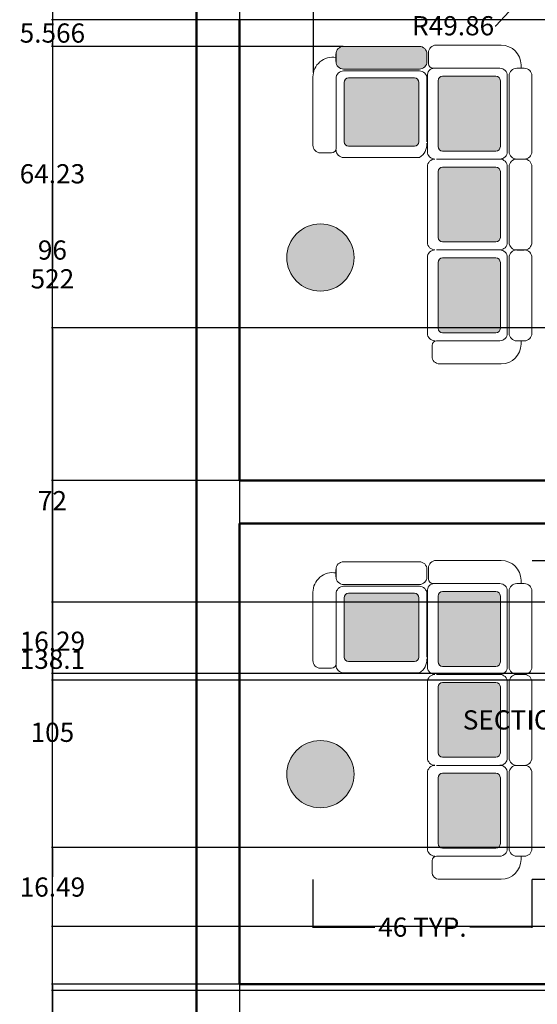
# Model space of a CAD drawing. Units: inches. Extents: x 1454 to 2136, y 626 to 1213.
# Tile 2 of 23: x 1456 to 1564, y 768 to 973. Entities that reach past the tile are written whole.
import ezdxf

# ---------------------------------------------------------------- set-up
doc = ezdxf.new("R2010")
doc.units = ezdxf.units.IN
doc.header["$MEASUREMENT"] = 0
for name, color, linetype, lineweight in [('A-ANNO-DIMS', 2, 'Continuous', 18), ('A-FURN', 9, 'Continuous', 18), ('A-FURN-PATT', 252, 'Continuous', 13), ('A-WALL', 7, 'Continuous', 50), ('sofa', 4, 'Continuous', 18)]:
    doc.layers.add(name, color=color, linetype=linetype, lineweight=lineweight)
doc.styles.get("Standard").update_dxf_attribs({"font": 'arial.ttf'})
doc.dimstyles.get("Standard").update_dxf_attribs({"dimtxt": 4, "dimasz": 0.18, "dimexe": 0.18, "dimexo": 0.0625, "dimgap": 0.09, "dimtad": 0, "dimtih": 1, "dimtoh": 1, "dimdec": 0, "dimrnd": 6, "dimzin": 0, "dimdsep": 46, "dimlunit": 3, "dimtxsty": 'Standard', "dimcen": 0.09, "dimadec": 0, "dimazin": 0, "dimtfac": 1, "dimtdec": 0, "dimtofl": 0, "dimtmove": 0, "dimatfit": 3, "dimfxl": 1, "dimtolj": 1, "dimtzin": 0, "dimarcsym": 0})

# ---------------------------------------------------------------- blocks, each defined once
blk = doc.blocks.new('A$C611E44E9')
for p, q in [((0.6611, 1.4447), (0.2101, 1.4447)), ((0.7111, 1.3223), (0.7111, 1.3947)), ((0.0084, 1.2424), (0.0084, 0.7424)), ((0.1084, 1.2927), (0.0584, 1.2927)), ((0.0584, 1.2924), (0.1084, 1.2924)), ((0.1584, 1.2424), (0.1584, 0.7424)), ((0.1705, 1.2422), (0.1705, 0.7424)), ((0.6811, 1.2924), (0.2205, 1.2924)), ((0.6811, 1.2924), (0.2205, 1.2924)), ((0.6811, 1.2922), (0.2205, 1.2922)), ((0.2465, 1.2392), (0.6374, 1.2392)), ((0.7418, 0.7424), (0.7418, 1.2422)), ((0.2165, 0.7749), (0.2165, 1.2092)), ((0.6674, 1.2092), (0.6674, 0.7749)), ((0.6374, 0.7449), (0.2465, 0.7449)), ((0.1224, 0.6827), (0.05, 0.6827)), ((0.1084, 0.6927), (0.0584, 0.6927)), ((0.0584, 0.6924), (0.1084, 0.6924)), ((0.1524, 0.6527), (0.1524, 0.2121)), ((0.2024, 0.6896), (0.7021, 0.6896)), ((0.6373, 0.6924), (0.2205, 0.6924)), ((0.6373, 0.6924), (0.2205, 0.6924)), ((0.8021, 0.6896), (1.3018, 0.6896)), ((1.4021, 0.6896), (1.9018, 0.6896)), ((1.982, 0.6589), (2.0543, 0.6589)), ((0, 0.6327), (0, 0.2017)), ((0.2048, 0.5892), (0.2048, 0.2381)), ((0.6691, 0.6192), (0.2348, 0.6192)), ((0.6991, 0.2381), (0.6991, 0.5892)), ((0.7521, 0.6289), (0.7521, 0.2121)), ((0.7521, 0.6289), (0.7521, 0.2121)), ((0.8045, 0.5892), (0.8045, 0.2381)), ((1.2688, 0.6192), (0.8345, 0.6192)), ((1.2988, 0.2381), (1.2988, 0.5892)), ((1.3521, 0.6289), (1.3521, 0.2121)), ((1.3521, 0.6289), (1.3521, 0.2121)), ((1.4045, 0.5892), (1.4045, 0.2381)), ((1.8688, 0.6192), (1.4345, 0.6192)), ((1.8988, 0.2381), (1.8988, 0.5892)), ((1.9518, 0.6289), (1.9518, 0.2121)), ((1.952, 0.6289), (1.952, 0.2121)), ((2.1043, 0.6089), (2.1043, 0.2017)), ((0.2348, 0.2081), (0.6691, 0.2081)), ((0.8345, 0.2081), (1.2688, 0.2081)), ((1.4345, 0.2081), (1.8688, 0.2081)), ((0.7021, 0.1621), (0.2024, 0.1621)), ((0.7024, 0.15), (0.2024, 0.15)), ((1.3018, 0.1621), (0.8021, 0.1621)), ((1.3021, 0.15), (0.8021, 0.15)), ((1.9018, 0.1621), (1.4021, 0.1621)), ((1.9021, 0.15), (1.4021, 0.15)), ((0.13, 0.0717), (0.15, 0.0717)), ((0.1524, 0.05), (0.1524, 0.1)), ((0.7521, 0.05), (0.7521, 0.1)), ((0.7524, 0.1), (0.7524, 0.05)), ((1.3521, 0.05), (1.3521, 0.1)), ((1.3524, 0.1), (1.3524, 0.05)), ((1.952, 0.05), (1.952, 0.1)), ((1.9521, 0.1), (1.9521, 0.05)), ((1.9743, 0.0717), (1.9543, 0.0717)), ((0.7024, 0), (0.2024, 0)), ((1.3021, 0), (0.8021, 0)), ((1.9021, 0), (1.4021, 0))]:
    blk.add_line(p, q)
for centre, radius, start, end in [((0.2101, 1.3147), 0.13, 90, 189.86144), ((0.6611, 1.3947), 0.05, 0, 90), ((0.6811, 1.3223), 0.03, 270, 0), ((0.0584, 1.2424), 0.05, 90, 180), ((0.1084, 1.2424), 0.05, 0, 90), ((0.2205, 1.2422), 0.05, 90, 180), ((0.2465, 1.2092), 0.03, 90, 180), ((0.6374, 1.2092), 0.03, 0, 90), ((0.6918, 1.2422), 0.05, 0, 90), ((0.0584, 0.7424), 0.05, 180, 270), ((0.1084, 0.7424), 0.05, 270, 0), ((0.2205, 0.7424), 0.05, 180, 270), ((0.2465, 0.7749), 0.03, 180, 270), ((0.6374, 0.7749), 0.03, 270, 0), ((0.653, 0.796), 0.1037, 267.24891, 328.87945), ((0.05, 0.6327), 0.05, 90, 180), ((0.1224, 0.6527), 0.03, 0, 90), ((0.1981, 0.6441), 0.0458, 84.66489, 178.99029), ((0.7021, 0.6396), 0.05, 0, 90), ((0.8021, 0.6396), 0.05, 90, 180), ((1.3018, 0.6396), 0.05, 0, 90), ((1.4021, 0.6396), 0.05, 90, 180), ((1.9018, 0.6396), 0.05, 0, 90), ((1.982, 0.6289), 0.03, 90, 180), ((2.0543, 0.6089), 0.05, 0, 90), ((0.2348, 0.5892), 0.03, 90, 180), ((0.6691, 0.5892), 0.03, 0, 90), ((0.8345, 0.5892), 0.03, 90, 180), ((1.2688, 0.5892), 0.03, 0, 90), ((1.4345, 0.5892), 0.03, 90, 180), ((1.8688, 0.5892), 0.03, 0, 90), ((0.13, 0.2017), 0.13, 180, 270), ((0.2024, 0.2121), 0.05, 180, 270), ((0.2348, 0.2381), 0.03, 180, 270), ((0.6691, 0.2381), 0.03, 270, 0), ((0.7021, 0.2121), 0.05, 270, 0), ((0.8021, 0.2121), 0.05, 180, 270), ((0.8345, 0.2381), 0.03, 180, 270), ((1.2688, 0.2381), 0.03, 270, 0), ((1.3018, 0.2121), 0.05, 270, 0), ((1.4021, 0.2121), 0.05, 180, 270), ((1.4345, 0.2381), 0.03, 180, 270), ((1.8688, 0.2381), 0.03, 270, 0), ((1.9018, 0.2121), 0.05, 270, 0), ((1.9743, 0.2017), 0.13, 270, 0), ((0.2024, 0.1), 0.05, 90, 180), ((0.7024, 0.1), 0.05, 0, 90), ((0.8021, 0.1), 0.05, 90, 180), ((1.3021, 0.1), 0.05, 0, 90), ((1.4021, 0.1), 0.05, 90, 180), ((1.9021, 0.1), 0.05, 0, 90), ((0.2024, 0.05), 0.05, 180, 270), ((0.7024, 0.05), 0.05, 270, 0), ((0.8021, 0.05), 0.05, 180, 270), ((1.3021, 0.05), 0.05, 270, 0), ((1.4021, 0.05), 0.05, 180, 270), ((1.9021, 0.05), 0.05, 270, 0)]:
    blk.add_arc(centre, radius, start, end)
blk = doc.blocks.new('*D13')
at = {"layer": 'A-ANNO-DIMS', "color": 0, "lineweight": -2, "transparency": 16777216}
for p, q in [((1562.49, 860.58), (1572.58, 860.58)), ((1572.4, 860.4), (1572.4, 829.52)), ((1572.4, 794.32), (1572.4, 825.2)), ((1562.49, 794.14), (1572.58, 794.14))]:
    blk.add_line(p, q, dxfattribs=at)
at = {"layer": 'A-ANNO-DIMS', "color": 0, "transparency": 16777216}
for points in [[(1572.37, 860.4), (1572.43, 860.4), (1572.4, 860.58)], [(1572.37, 794.32), (1572.43, 794.32), (1572.4, 794.14)]]:
    blk.add_solid(points, dxfattribs=at)
at = {"layer": 'Defpoints', "color": 0, "transparency": 16777216}
for p in [(1562.43, 860.58), (1562.43, 794.14), (1572.4, 794.14)]:
    blk.add_point(p, dxfattribs=at)
at = {"layer": 'A-ANNO-DIMS', "color": 0, "transparency": 16777216, "insert": (1572.4, 827.36), "char_height": 4, "attachment_point": 5}
blk.add_mtext('\\A1;SECTIONAL 66 TYP.', dxfattribs=at)
blk = doc.blocks.new('*D14')
at = {"layer": 'A-ANNO-DIMS', "color": 0, "lineweight": -2, "transparency": 16777216}
for p, q in [((1516.82, 794.08), (1516.82, 784)), ((1562.43, 794.08), (1562.43, 784)), ((1517, 784.18), (1529.72, 784.18)), ((1562.25, 784.18), (1549.53, 784.18))]:
    blk.add_line(p, q, dxfattribs=at)
at = {"layer": 'A-ANNO-DIMS', "color": 0, "transparency": 16777216}
for points in [[(1517, 784.21), (1517, 784.15), (1516.82, 784.18)], [(1562.25, 784.21), (1562.25, 784.15), (1562.43, 784.18)]]:
    blk.add_solid(points, dxfattribs=at)
at = {"layer": 'Defpoints', "color": 0, "transparency": 16777216}
for p in [(1516.82, 794.14), (1562.43, 794.14), (1516.82, 784.18)]:
    blk.add_point(p, dxfattribs=at)
at = {"layer": 'A-ANNO-DIMS', "color": 0, "transparency": 16777216, "insert": (1539.63, 784.18), "char_height": 4, "attachment_point": 5}
blk.add_mtext('\\A1;46 TYP.', dxfattribs=at)
blk = doc.blocks.new('*D28')
at = {"layer": 'A-ANNO-DIMS', "color": 0, "lineweight": -2, "transparency": 16777216}
for p, q in [((1537.49, 1180.28), (1462.37, 1180.28)), ((1462.55, 1180.1), (1462.55, 921.41)), ((1462.55, 658.46), (1462.55, 917.15)), ((1492.49, 658.28), (1462.37, 658.28))]:
    blk.add_line(p, q, dxfattribs=at)
at = {"layer": 'A-ANNO-DIMS', "color": 0, "transparency": 16777216}
for points in [[(1462.52, 1180.1), (1462.58, 1180.1), (1462.55, 1180.28)], [(1462.52, 658.46), (1462.58, 658.46), (1462.55, 658.28)]]:
    blk.add_solid(points, dxfattribs=at)
at = {"layer": 'Defpoints', "color": 0, "transparency": 16777216}
for p in [(1462.55, 1180.28), (1537.56, 1180.28), (1492.56, 658.28)]:
    blk.add_point(p, dxfattribs=at)
at = {"layer": 'A-ANNO-DIMS', "color": 0, "transparency": 16777216, "insert": (1462.55, 919.28), "char_height": 4, "attachment_point": 5}
blk.add_mtext('\\A1;522', dxfattribs=at)
blk = doc.blocks.new('*D40')
at = {"layer": 'A-ANNO-DIMS', "color": 0, "lineweight": -2, "transparency": 16777216}
for p, q in [((1501.56, 877.34), (1501.56, 1210.46)), ((1501.74, 1210.28), (1569.24, 1210.28)), ((1645.38, 1210.28), (1577.87, 1210.28)), ((1645.56, 877.34), (1645.56, 1210.46))]:
    blk.add_line(p, q, dxfattribs=at)
at = {"layer": 'A-ANNO-DIMS', "color": 0, "transparency": 16777216}
for points in [[(1501.74, 1210.31), (1501.74, 1210.25), (1501.56, 1210.28)], [(1645.38, 1210.31), (1645.38, 1210.25), (1645.56, 1210.28)]]:
    blk.add_solid(points, dxfattribs=at)
at = {"layer": 'Defpoints', "color": 0, "transparency": 16777216}
for p in [(1645.56, 1210.28), (1501.56, 877.28), (1645.56, 877.28)]:
    blk.add_point(p, dxfattribs=at)
at = {"layer": 'A-ANNO-DIMS', "color": 0, "transparency": 16777216, "insert": (1573.56, 1210.28), "char_height": 4, "attachment_point": 5}
blk.add_mtext('\\A1;144', dxfattribs=at)
blk = doc.blocks.new('*D41')
at = {"layer": 'A-ANNO-DIMS', "color": 0, "lineweight": -2, "transparency": 16777216}
for p, q in [((1645.49, 772.28), (1462.37, 772.28)), ((1462.55, 772.1), (1462.55, 721.91)), ((1462.55, 667.46), (1462.55, 717.65)), ((1645.49, 667.28), (1462.37, 667.28))]:
    blk.add_line(p, q, dxfattribs=at)
at = {"layer": 'A-ANNO-DIMS', "color": 0, "transparency": 16777216}
for points in [[(1462.52, 772.1), (1462.58, 772.1), (1462.55, 772.28)], [(1462.52, 667.46), (1462.58, 667.46), (1462.55, 667.28)]]:
    blk.add_solid(points, dxfattribs=at)
at = {"layer": 'Defpoints', "color": 0, "transparency": 16777216}
for p in [(1462.55, 772.28), (1645.56, 772.28), (1645.56, 667.28)]:
    blk.add_point(p, dxfattribs=at)
at = {"layer": 'A-ANNO-DIMS', "color": 0, "transparency": 16777216, "insert": (1462.55, 719.78), "char_height": 4, "attachment_point": 5}
blk.add_mtext('\\A1;105', dxfattribs=at)
blk = doc.blocks.new('*D42')
at = {"layer": 'A-ANNO-DIMS', "color": 0, "lineweight": -2, "transparency": 16777216}
for p, q in [((1645.49, 877.28), (1462.37, 877.28)), ((1462.55, 877.1), (1462.55, 826.91)), ((1462.55, 772.46), (1462.55, 822.65)), ((1645.49, 772.28), (1462.37, 772.28))]:
    blk.add_line(p, q, dxfattribs=at)
at = {"layer": 'A-ANNO-DIMS', "color": 0, "transparency": 16777216}
for points in [[(1462.52, 877.1), (1462.58, 877.1), (1462.55, 877.28)], [(1462.52, 772.46), (1462.58, 772.46), (1462.55, 772.28)]]:
    blk.add_solid(points, dxfattribs=at)
at = {"layer": 'Defpoints', "color": 0, "transparency": 16777216}
for p in [(1462.55, 877.28), (1645.56, 877.28), (1645.56, 772.28)]:
    blk.add_point(p, dxfattribs=at)
at = {"layer": 'A-ANNO-DIMS', "color": 0, "transparency": 16777216, "insert": (1462.55, 824.78), "char_height": 4, "attachment_point": 5}
blk.add_mtext('\\A1;105', dxfattribs=at)
blk = doc.blocks.new('*D43')
at = {"layer": 'A-ANNO-DIMS', "color": 0, "lineweight": -2, "transparency": 16777216}
for p, q in [((1501.49, 973.28), (1462.37, 973.28)), ((1462.55, 973.1), (1462.55, 927.41)), ((1462.55, 877.46), (1462.55, 923.15)), ((1501.49, 877.28), (1462.37, 877.28))]:
    blk.add_line(p, q, dxfattribs=at)
at = {"layer": 'A-ANNO-DIMS', "color": 0, "transparency": 16777216}
for points in [[(1462.52, 973.1), (1462.58, 973.1), (1462.55, 973.28)], [(1462.52, 877.46), (1462.58, 877.46), (1462.55, 877.28)]]:
    blk.add_solid(points, dxfattribs=at)
at = {"layer": 'Defpoints', "color": 0, "transparency": 16777216}
for p in [(1462.55, 973.28), (1501.56, 973.28), (1501.56, 877.28)]:
    blk.add_point(p, dxfattribs=at)
at = {"layer": 'A-ANNO-DIMS', "color": 0, "transparency": 16777216, "insert": (1462.55, 925.28), "char_height": 4, "attachment_point": 5}
blk.add_mtext('\\A1;96', dxfattribs=at)
blk = doc.blocks.new('*D46')
at = {"layer": 'A-ANNO-DIMS', "color": 0, "lineweight": -2, "transparency": 16777216}
for p, q in [((1701.01, 909.05), (1462.37, 909.05)), ((1462.55, 908.87), (1462.55, 842.13)), ((1462.55, 771.13), (1462.55, 837.86)), ((1753.01, 770.95), (1462.37, 770.95))]:
    blk.add_line(p, q, dxfattribs=at)
at = {"layer": 'A-ANNO-DIMS', "color": 0, "transparency": 16777216}
for points in [[(1462.52, 908.87), (1462.58, 908.87), (1462.55, 909.05)], [(1462.52, 771.13), (1462.58, 771.13), (1462.55, 770.95)]]:
    blk.add_solid(points, dxfattribs=at)
at = {"layer": 'Defpoints', "color": 0, "transparency": 16777216}
for p in [(1701.08, 909.05), (1462.55, 770.95), (1753.08, 770.95)]:
    blk.add_point(p, dxfattribs=at)
at = {"layer": 'A-ANNO-DIMS', "color": 0, "transparency": 16777216, "insert": (1462.55, 840), "char_height": 4, "attachment_point": 5}
blk.add_mtext('\\A1;138.1', dxfattribs=at)
blk = doc.blocks.new('*D48')
at = {"layer": 'A-ANNO-DIMS', "color": 0, "lineweight": -2, "transparency": 16777216}
for p, q in [((1879.49, 973.28), (1462.37, 973.28)), ((1462.55, 973.1), (1462.55, 943.3)), ((1462.55, 909.23), (1462.55, 939.03)), ((1885.19, 909.05), (1462.37, 909.05))]:
    blk.add_line(p, q, dxfattribs=at)
at = {"layer": 'A-ANNO-DIMS', "color": 0, "transparency": 16777216}
for points in [[(1462.52, 973.1), (1462.58, 973.1), (1462.55, 973.28)], [(1462.52, 909.23), (1462.58, 909.23), (1462.55, 909.05)]]:
    blk.add_solid(points, dxfattribs=at)
at = {"layer": 'Defpoints', "color": 0, "transparency": 16777216}
for p in [(1879.56, 973.28), (1462.55, 909.05), (1885.25, 909.05)]:
    blk.add_point(p, dxfattribs=at)
at = {"layer": 'A-ANNO-DIMS', "color": 0, "transparency": 16777216, "insert": (1462.55, 941.17), "char_height": 4, "attachment_point": 5}
blk.add_mtext('\\A1;64.23', dxfattribs=at)
blk = doc.blocks.new('*D52')
at = {"layer": 'A-ANNO-DIMS', "color": 0, "lineweight": -2, "transparency": 16777216}
for p, q in [((1927.57, 800.77), (1462.37, 800.77)), ((1462.55, 800.59), (1462.55, 794.66)), ((1462.55, 784.46), (1462.55, 790.4)), ((1927.49, 784.28), (1462.37, 784.28))]:
    blk.add_line(p, q, dxfattribs=at)
at = {"layer": 'A-ANNO-DIMS', "color": 0, "transparency": 16777216}
for points in [[(1462.52, 800.59), (1462.58, 800.59), (1462.55, 800.77)], [(1462.52, 784.46), (1462.58, 784.46), (1462.55, 784.28)]]:
    blk.add_solid(points, dxfattribs=at)
at = {"layer": 'Defpoints', "color": 0, "transparency": 16777216}
for p in [(1462.55, 800.77), (1927.64, 800.77), (1927.56, 784.28)]:
    blk.add_point(p, dxfattribs=at)
at = {"layer": 'A-ANNO-DIMS', "color": 0, "transparency": 16777216, "insert": (1462.55, 792.53), "char_height": 4, "attachment_point": 5}
blk.add_mtext('\\A1;16.49', dxfattribs=at)
blk = doc.blocks.new('*D53')
at = {"layer": 'A-ANNO-DIMS', "color": 0, "lineweight": -2, "transparency": 16777216}
for p, q in [((1927.57, 851.9), (1462.37, 851.9)), ((1462.55, 851.72), (1462.55, 845.89)), ((1462.55, 835.79), (1462.55, 841.63)), ((1927.57, 835.61), (1462.37, 835.61))]:
    blk.add_line(p, q, dxfattribs=at)
at = {"layer": 'A-ANNO-DIMS', "color": 0, "transparency": 16777216}
for points in [[(1462.52, 851.72), (1462.58, 851.72), (1462.55, 851.9)], [(1462.52, 835.79), (1462.58, 835.79), (1462.55, 835.61)]]:
    blk.add_solid(points, dxfattribs=at)
at = {"layer": 'Defpoints', "color": 0, "transparency": 16777216}
for p in [(1462.55, 851.9), (1927.64, 851.9), (1927.64, 835.61)]:
    blk.add_point(p, dxfattribs=at)
at = {"layer": 'A-ANNO-DIMS', "color": 0, "transparency": 16777216, "insert": (1462.55, 843.76), "char_height": 4, "attachment_point": 5}
blk.add_mtext('\\A1;16.29', dxfattribs=at)
blk = doc.blocks.new('*D65')
at = {"layer": 'A-ANNO-DIMS', "color": 0, "lineweight": -2, "transparency": 16777216}
for p, q in [((1885.19, 909.05), (1462.37, 909.05)), ((1462.55, 908.87), (1462.55, 875.15)), ((1462.55, 837.23), (1462.55, 870.95)), ((1885.19, 837.05), (1462.37, 837.05))]:
    blk.add_line(p, q, dxfattribs=at)
at = {"layer": 'A-ANNO-DIMS', "color": 0, "transparency": 16777216}
for points in [[(1462.52, 908.87), (1462.58, 908.87), (1462.55, 909.05)], [(1462.52, 837.23), (1462.58, 837.23), (1462.55, 837.05)]]:
    blk.add_solid(points, dxfattribs=at)
at = {"layer": 'Defpoints', "color": 0, "transparency": 16777216}
for p in [(1885.25, 909.05), (1462.55, 837.05), (1885.25, 837.05)]:
    blk.add_point(p, dxfattribs=at)
at = {"layer": 'A-ANNO-DIMS', "color": 0, "transparency": 16777216, "insert": (1462.55, 873.05), "char_height": 4, "attachment_point": 5}
blk.add_mtext('\\A1;72', dxfattribs=at)
blk = doc.blocks.new('*D79')
at = {"layer": 'A-ANNO-DIMS', "color": 0, "lineweight": -2, "transparency": 16777216}
for p, q in [((1501.56, 973.34), (1501.56, 1210.46)), ((1501.74, 1210.28), (1516.74, 1210.28)), ((1516.92, 962.3), (1516.92, 1210.46)), ((1516.92, 1210.28), (1517.1, 1210.28))]:
    blk.add_line(p, q, dxfattribs=at)
at = {"layer": 'A-ANNO-DIMS', "color": 0, "transparency": 16777216}
for points in [[(1501.74, 1210.31), (1501.74, 1210.25), (1501.56, 1210.28)], [(1516.74, 1210.31), (1516.74, 1210.25), (1516.92, 1210.28)]]:
    blk.add_solid(points, dxfattribs=at)
at = {"layer": 'Defpoints', "color": 0, "transparency": 16777216}
for p in [(1516.92, 1210.28), (1501.56, 973.28), (1516.92, 962.24)]:
    blk.add_point(p, dxfattribs=at)
at = {"layer": 'A-ANNO-DIMS', "color": 0, "transparency": 16777216, "insert": (1525.28, 1210.28), "char_height": 4, "attachment_point": 5}
blk.add_mtext('\\A1;15.362', dxfattribs=at)
blk = doc.blocks.new('*D80')
at = {"layer": 'A-ANNO-DIMS', "color": 0, "lineweight": -2, "transparency": 16777216}
for p, q in [((1501.49, 973.28), (1462.37, 973.28)), ((1462.55, 973.1), (1462.55, 972.63)), ((1523.14, 967.72), (1462.37, 967.72)), ((1462.55, 967.9), (1462.55, 968.37))]:
    blk.add_line(p, q, dxfattribs=at)
at = {"layer": 'A-ANNO-DIMS', "color": 0, "transparency": 16777216}
for points in [[(1462.52, 973.1), (1462.58, 973.1), (1462.55, 973.28)], [(1462.52, 967.9), (1462.58, 967.9), (1462.55, 967.72)]]:
    blk.add_solid(points, dxfattribs=at)
at = {"layer": 'Defpoints', "color": 0, "transparency": 16777216}
for p in [(1501.56, 973.28), (1462.55, 967.72), (1523.21, 967.72)]:
    blk.add_point(p, dxfattribs=at)
at = {"layer": 'A-ANNO-DIMS', "color": 0, "transparency": 16777216, "insert": (1462.55, 970.5), "char_height": 4, "attachment_point": 5}
blk.add_mtext('\\A1;5.566', dxfattribs=at)
blk = doc.blocks.new('*D88')
at = {"layer": 'A-ANNO-DIMS', "color": 0, "lineweight": -2, "transparency": 16777216}
for p, q in [((1492.56, 658.34), (1492.56, 1210.46)), ((1492.74, 1210.28), (1495.65, 1210.28)), ((1501.38, 1210.28), (1498.46, 1210.28)), ((1501.56, 667.34), (1501.56, 1210.46))]:
    blk.add_line(p, q, dxfattribs=at)
at = {"layer": 'A-ANNO-DIMS', "color": 0, "transparency": 16777216}
for points in [[(1492.74, 1210.31), (1492.74, 1210.25), (1492.56, 1210.28)], [(1501.38, 1210.31), (1501.38, 1210.25), (1501.56, 1210.28)]]:
    blk.add_solid(points, dxfattribs=at)
at = {"layer": 'Defpoints', "color": 0, "transparency": 16777216}
for p in [(1501.56, 1210.28), (1501.56, 667.28), (1492.56, 658.28)]:
    blk.add_point(p, dxfattribs=at)
at = {"layer": 'A-ANNO-DIMS', "color": 0, "transparency": 16777216, "insert": (1497.06, 1210.28), "char_height": 4, "attachment_point": 5}
blk.add_mtext('\\A1;9', dxfattribs=at)
blk = doc.blocks.new('*D92')
at = {"layer": 'A-ANNO-DIMS', "color": 0, "lineweight": -2, "transparency": 16777216}
for p, q in [((1608.77, 1030.83), (1608.95, 1030.83)), ((1608.86, 1030.74), (1608.86, 1030.92)), ((1554.95, 972.02), (1575.05, 993.94)), ((1554.77, 972.02), (1554.95, 972.02))]:
    blk.add_line(p, q, dxfattribs=at)
at = {"layer": 'A-ANNO-DIMS', "color": 0, "transparency": 16777216}
blk.add_solid([(1575.02, 993.96), (1575.07, 993.92), (1575.17, 994.07)], dxfattribs=at)
at = {"layer": 'Defpoints', "color": 0, "transparency": 16777216}
for p in [(1608.86, 1030.83), (1575.17, 994.07)]:
    blk.add_point(p, dxfattribs=at)
at = {"layer": 'A-ANNO-DIMS', "color": 0, "transparency": 16777216, "insert": (1546.02, 972.02), "char_height": 4, "attachment_point": 5}
blk.add_mtext('\\A1;R49.86', dxfattribs=at)

msp = doc.modelspace()

# ---------------------------------------------------------------- hatches: boundary and pattern name
at = {"layer": 'A-FURN-PATT'}
h = msp.add_hatch(dxfattribs=at)
h.set_pattern_fill('ESCHER', color=256)
h.paths.add_polyline_path([(1511.3761, 923.7174, 1), (1525.379, 923.7174, 1)])
h.paths.add_polyline_path([(1525.379, 816.0542, 1), (1511.3761, 816.0542, 1)])
h.paths.add_polyline_path([(1525.379, 712.7345, 1), (1511.3761, 712.7345, 1)])
h.paths.add_polyline_path([(2070.5057, 794.3402, 1), (2056.5027, 794.3402, 1)])
h.paths.add_polyline_path([(2005.868, 1014.5578, 1), (1991.8651, 1014.5578, 1)])
h.paths.add_polyline_path([(1994.0647, 1066.7584, 1), (2008.0677, 1066.7584, 1)])
h.paths.add_polyline_path([(1919.5492, 1065.3848, 1), (1933.5521, 1065.3848, 1)])
h.paths.add_polyline_path([(1936.8517, 1013.7336, 1), (1922.8488, 1013.7336, 1)])
h.paths.add_polyline_path([(1824.6062, 1109.1557, 1), (1838.6091, 1109.1557, 1)])
h = msp.add_hatch(color=256, dxfattribs=at)
h.dxf.hatch_style = 1
h.paths.add_polyline_path([(1855.0231, 1089.5248, 0.41421356), (1850.0231, 1094.5248), (1811.2288, 1094.5248, 0.41421356), (1806.2288, 1089.5248), (1806.2288, 1083.6305, 0.41421356), (1811.2288, 1078.6305), (1850.0231, 1078.6305, 0.41421356), (1855.0231, 1083.6305)])
h.paths.add_polyline_path([(1939.0638, 1089.4209), (1938.9354, 1078.7354, -0.20858653), (1943.5258, 1076.1857), (1952.7682, 1081.5837, 0.24238954)])
h.paths.add_polyline_path([(1939.0638, 1089.4209, 0.00796483), (1938.5148, 1089.4363), (1928.0643, 1089.5619), (1927.936, 1078.8906), (1938.3866, 1078.765, -0.02092855), (1938.9354, 1078.7354)])
h.paths.add_polyline_path([(1928.0643, 1089.5619), (1916.0797, 1089.706), (1916.0698, 1088.8851), (1917.241, 1088.8711, -0.41420041), (1917.7276, 1088.3726), (1917.6308, 1080.3281, -0.41422672), (1917.1324, 1079.8415), (1915.9612, 1079.8556), (1915.9573, 1079.5272, 0.41420799), (1916.4439, 1079.0288), (1927.936, 1078.8906)])
h.paths.add_polyline_path([(1917.7276, 1088.3726, 0.41420041), (1917.241, 1088.8711), (1914.9926, 1088.8981, 0.41421356), (1914.4941, 1088.4115), (1914.3974, 1080.367, 0.41421356), (1914.884, 1079.8686), (1917.1324, 1079.8415, 0.41422672), (1917.6308, 1080.3281)])
h.paths.add_polyline_path([(1928.0939, 1092.0245), (1916.6018, 1092.1627, 0.41422672), (1916.1033, 1091.6761), (1916.0797, 1089.706), (1928.0643, 1089.5619)])
h.paths.add_polyline_path([(1939.0935, 1091.8846, 0.00696804), (1938.5445, 1091.8989), (1928.0939, 1092.0245), (1928.0643, 1089.5619), (1938.5148, 1089.4363, -0.00796483), (1939.0638, 1089.4209)])
h.paths.add_polyline_path([(1939.0935, 1091.8846), (1939.0638, 1089.4209, -0.24238954), (1952.7682, 1081.5837), (1954.897, 1082.827, 0.24500473)])
h.paths.add_polyline_path([(1952.7682, 1081.5837), (1943.5258, 1076.1857, -0.16768112), (1944.8746, 1072.1191), (1944.8073, 1066.5201), (1955.4785, 1066.3918), (1955.5459, 1071.9909, 0.14799784)])
h.paths.add_polyline_path([(1954.897, 1082.827), (1952.7682, 1081.5837, -0.14799784), (1955.5459, 1071.9909), (1955.4785, 1066.3918), (1957.9412, 1066.3622), (1958.0085, 1071.9612, 0.14649407)])
h.paths.add_polyline_path([(1955.4785, 1066.3918), (1944.8073, 1066.5201), (1944.675, 1055.5205, 0.41421356), (1945.1616, 1055.0221), (1945.49, 1055.0181), (1945.5041, 1056.1893, -0.41421356), (1946.0025, 1056.6759), (1954.047, 1056.5792, -0.41421356), (1954.5336, 1056.0807), (1954.5195, 1054.9096), (1955.3404, 1054.8997)])
h.paths.add_polyline_path([(1954.5336, 1056.0807, 0.41421356), (1954.047, 1056.5792), (1946.0025, 1056.6759, 0.41421356), (1945.5041, 1056.1893), (1945.49, 1055.0181), (1945.477, 1053.9409, 0.41422115), (1945.9636, 1053.4425), (1954.0081, 1053.3458, 0.41420598), (1954.5066, 1053.8324)])
h.paths.add_polyline_path([(1957.9412, 1066.3622), (1955.4785, 1066.3918), (1955.3404, 1054.8997), (1957.3105, 1054.876, 0.41421356), (1957.8089, 1055.3626)])
h.paths.add_polyline_path([(1974.6911, 1066.3918), (1972.2285, 1066.3622), (1972.3608, 1055.3626, 0.41421356), (1972.8592, 1054.876), (1974.8293, 1054.8997)])
h.paths.add_polyline_path([(1985.3624, 1066.5201), (1974.6911, 1066.3918), (1974.8293, 1054.8997), (1975.6501, 1054.9096), (1975.6361, 1056.0807, -0.41421356), (1976.1227, 1056.5792), (1984.1672, 1056.6759, -0.41421356), (1984.6656, 1056.1893), (1984.6797, 1055.0181), (1985.008, 1055.0221, 0.41421356), (1985.4946, 1055.5205)])
h.paths.add_polyline_path([(1984.6656, 1056.1893, 0.41421356), (1984.1672, 1056.6759), (1976.1227, 1056.5792, 0.41421356), (1975.6361, 1056.0807), (1975.6631, 1053.8324, 0.41422115), (1976.1615, 1053.3458), (1984.206, 1053.4425, 0.41420597), (1984.6926, 1053.9409)])
h.paths.add_polyline_path([(1985.2951, 1072.1191, -0.16768112), (1986.6438, 1076.1857), (1977.4014, 1081.5837, 0.14799988), (1974.6238, 1071.9907), (1974.6911, 1066.3918), (1985.3624, 1066.5201)])
h.paths.add_polyline_path([(1977.4014, 1081.5837), (1975.2727, 1082.827, 0.14649407), (1972.1612, 1071.9612), (1972.2285, 1066.3622), (1974.6911, 1066.3918), (1974.6238, 1071.9907, -0.14799988)])
h.paths.add_polyline_path([(1991.1058, 1089.4209, 0.24238954), (1977.4014, 1081.5837), (1986.6438, 1076.1857, -0.20858653), (1991.2343, 1078.7354)])
h.paths.add_polyline_path([(1991.1058, 1089.4209), (1991.0762, 1091.8846, 0.24500473), (1975.2727, 1082.827), (1977.4014, 1081.5837, -0.24238954)])
h.paths.add_polyline_path([(2002.1053, 1089.5619), (1991.6547, 1089.4363, 0.00796283), (1991.1058, 1089.4209), (1991.2343, 1078.7354, -0.02092855), (1991.783, 1078.765), (2002.2336, 1078.8906)])
h.paths.add_polyline_path([(2002.0757, 1092.0245), (1991.6251, 1091.8989, 0.00696804), (1991.0762, 1091.8846), (1991.1058, 1089.4209, -0.00796283), (1991.6547, 1089.4363), (2002.1053, 1089.5619)])
h.paths.add_polyline_path([(2014.0663, 1091.6761, 0.4142004), (2013.5679, 1092.1627), (2002.0757, 1092.0245), (2002.1053, 1089.5619), (2014.09, 1089.706)])
h.paths.add_polyline_path([(2012.4421, 1088.3726, -0.41422672), (2012.9287, 1088.8711), (2014.0999, 1088.8851), (2014.09, 1089.706), (2002.1053, 1089.5619), (2002.2336, 1078.8906), (2013.7258, 1079.0288, 0.41421913), (2014.2124, 1079.5273), (2014.2084, 1079.8556), (2013.0373, 1079.8415, -0.4142004), (2012.5388, 1080.3281)])
h.paths.add_polyline_path([(1986.6438, 1024.0964), (1977.4014, 1029.4944, 0.14799988), (1974.6238, 1019.9014), (1974.6911, 1014.3025), (1985.3624, 1014.4308), (1985.2951, 1020.0298, -0.16768112)])
h.paths.add_polyline_path([(1991.1058, 1037.3316, 0.24238954), (1977.4014, 1029.4944), (1986.6438, 1024.0964, -0.20858653), (1991.2343, 1026.6461)])
h.paths.add_polyline_path([(2002.1053, 1037.4726), (1991.6547, 1037.347, 0.00796283), (1991.1058, 1037.3316), (1991.2343, 1026.6461, -0.02092855), (1991.783, 1026.6757), (2002.2336, 1026.8013)])
h.paths.add_polyline_path([(2012.4421, 1036.2833, -0.41422672), (2012.9287, 1036.7818), (2014.0999, 1036.7958), (2014.09, 1037.6167), (2002.1053, 1037.4726), (2002.2336, 1026.8013), (2013.7258, 1026.9395, 0.41421913), (2014.2124, 1027.438), (2014.2084, 1027.7663), (2013.0373, 1027.7522, -0.4142004), (2012.5388, 1028.2388)])
h.paths.add_polyline_path([(2015.6755, 1036.3222, 0.41421356), (2015.1771, 1036.8088), (2012.9287, 1036.7818, 0.41422672), (2012.4421, 1036.2833), (2012.5388, 1028.2388, 0.4142004), (2013.0373, 1027.7522), (2015.2856, 1027.7793, 0.41421356), (2015.7722, 1028.2777)])
h.paths.add_polyline_path([(1985.3624, 1014.4308), (1974.6911, 1014.3025), (1974.8293, 1002.8104), (1975.6501, 1002.8203), (1975.6361, 1003.9914, -0.41421356), (1976.1227, 1004.4899), (1984.1672, 1004.5866, -0.41421356), (1984.6656, 1004.1), (1984.6797, 1002.9288), (1985.008, 1002.9328, 0.41421356), (1985.4946, 1003.4312)])
h.paths.add_polyline_path([(1984.6656, 1004.1, 0.41421356), (1984.1672, 1004.5866), (1976.1227, 1004.4899, 0.41421356), (1975.6361, 1003.9914), (1975.6631, 1001.743, 0.41422115), (1976.1615, 1001.2564), (1984.206, 1001.3532, 0.41420598), (1984.6926, 1001.8516)])
h.paths.add_polyline_path([(1974.6911, 1014.3025), (1972.2285, 1014.2729), (1972.3608, 1003.2733, 0.41421356), (1972.8592, 1002.7867), (1974.8293, 1002.8104)])
h.paths.add_polyline_path([(1974.6238, 1019.9014, -0.14799988), (1977.4014, 1029.4944), (1975.2727, 1030.7376, 0.14649407), (1972.1612, 1019.8719), (1972.2285, 1014.2729), (1974.6911, 1014.3025)])
h.paths.add_polyline_path([(1991.1058, 1037.3316), (1991.0762, 1039.7953, 0.24500473), (1975.2727, 1030.7376), (1977.4014, 1029.4944, -0.24238954)])
h.paths.add_polyline_path([(2002.0757, 1039.9352), (1991.6251, 1039.8096, 0.00696804), (1991.0762, 1039.7953), (1991.1058, 1037.3316, -0.00796283), (1991.6547, 1037.347), (2002.1053, 1037.4726)])
h.paths.add_polyline_path([(2014.0663, 1039.5868, 0.4142004), (2013.5679, 1040.0734), (2002.0757, 1039.9352), (2002.1053, 1037.4726), (2014.09, 1037.6167)])
h.paths.add_polyline_path([(1955.5459, 1019.9016, 0.14799784), (1952.7682, 1029.4944), (1943.5258, 1024.0964, -0.16768112), (1944.8746, 1020.0298), (1944.8073, 1014.4308), (1955.4785, 1014.3025)])
h.paths.add_polyline_path([(1955.4785, 1014.3025), (1944.8073, 1014.4308), (1944.675, 1003.4312, 0.41421356), (1945.1616, 1002.9328), (1945.49, 1002.9288), (1945.5041, 1004.1, -0.41421356), (1946.0025, 1004.5866), (1954.047, 1004.4899, -0.41421356), (1954.5336, 1003.9914), (1954.5195, 1002.8203), (1955.3404, 1002.8104)])
h.paths.add_polyline_path([(1939.0638, 1037.3316), (1938.9354, 1026.6461, -0.20858653), (1943.5258, 1024.0964), (1952.7682, 1029.4944, 0.24238954)])
h.paths.add_polyline_path([(1939.0638, 1037.3316, 0.00796483), (1938.5148, 1037.347), (1928.0643, 1037.4726), (1927.936, 1026.8013), (1938.3866, 1026.6757, -0.02092855), (1938.9354, 1026.6461)])
h.paths.add_polyline_path([(1928.0643, 1037.4726), (1916.0797, 1037.6167), (1916.0698, 1036.7958), (1917.241, 1036.7818, -0.41420041), (1917.7276, 1036.2833), (1917.6308, 1028.2388, -0.41422672), (1917.1324, 1027.7522), (1915.9612, 1027.7663), (1915.9573, 1027.4379, 0.41420799), (1916.4439, 1026.9395), (1927.936, 1026.8013)])
h.paths.add_polyline_path([(1917.7276, 1036.2833, 0.41420041), (1917.241, 1036.7818), (1914.9926, 1036.8088, 0.41421356), (1914.4941, 1036.3222), (1914.3974, 1028.2777, 0.41421356), (1914.884, 1027.7793), (1917.1324, 1027.7522, 0.41422672), (1917.6308, 1028.2388)])
h.paths.add_polyline_path([(1928.0939, 1039.9352), (1916.6018, 1040.0734, 0.41422672), (1916.1033, 1039.5868), (1916.0797, 1037.6167), (1928.0643, 1037.4726)])
h.paths.add_polyline_path([(1939.0935, 1039.7953, 0.00696804), (1938.5445, 1039.8096), (1928.0939, 1039.9352), (1928.0643, 1037.4726), (1938.5148, 1037.347, -0.00796483), (1939.0638, 1037.3316)])
h.paths.add_polyline_path([(1939.0935, 1039.7953), (1939.0638, 1037.3316, -0.24238954), (1952.7682, 1029.4944), (1954.897, 1030.7376, 0.24500473)])
h.paths.add_polyline_path([(1954.897, 1030.7376), (1952.7682, 1029.4944, -0.14799784), (1955.5459, 1019.9016), (1955.4785, 1014.3025), (1957.9412, 1014.2729), (1958.0085, 1019.8719, 0.14649407)])
h.paths.add_polyline_path([(1957.9412, 1014.2729), (1955.4785, 1014.3025), (1955.3404, 1002.8104), (1957.3105, 1002.7867, 0.41421356), (1957.8089, 1003.2733)])
h.paths.add_polyline_path([(1954.5336, 1003.9914, 0.41421356), (1954.047, 1004.4899), (1946.0025, 1004.5866, 0.41421356), (1945.5041, 1004.1), (1945.49, 1002.9288), (1945.477, 1001.8516, 0.41422115), (1945.9636, 1001.3532), (1954.0081, 1001.2564, 0.41420598), (1954.5066, 1001.743)])
h.paths.add_polyline_path([(1997.553, 886.9384), (1981.0334, 886.9384), (1981.0334, 876.3409, 0.41421356), (1984.1503, 873.224), (1996.6179, 873.224, 0.41421356), (1999.7348, 876.3409), (1998.488, 876.3409, -0.41421356), (1997.553, 877.276)])
h.paths.add_polyline_path([(1981.0334, 886.9384), (1964.5139, 886.9384), (1964.5139, 877.276, -0.41421356), (1963.5788, 876.3409), (1962.3321, 876.3409, 0.41421356), (1965.449, 873.224), (1977.9165, 873.224, 0.41421356), (1981.0334, 876.3409)])
h.paths.add_polyline_path([(1964.5139, 886.9384), (1964.5139, 887.25, 0.47353022), (1963.4209, 888.1978, -0.46345458), (1962.3321, 889.1202), (1962.3321, 890.6786), (1962.3321, 892.5488), (1961.0853, 892.5488, 0.41421356), (1960.1503, 891.6137), (1960.1503, 877.276, 0.41421356), (1961.0853, 876.3409), (1963.5788, 876.3409, 0.41421356), (1964.5139, 877.276)])
h.paths.add_polyline_path([(1999.7348, 892.5488), (1999.7348, 893.7955, 0.41421356), (1998.7997, 894.7306), (1963.2672, 894.7306, 0.41421356), (1962.3321, 893.7955), (1962.3321, 892.5488), (1962.3321, 890.3669, 0.41421356), (1963.2672, 889.4319), (1998.7997, 889.4319, 0.41421356), (1999.7348, 890.3669), (1999.7348, 890.6786)])
h.paths.add_polyline_path([(2001.9166, 891.6137, 0.41421356), (2000.9815, 892.5488), (1999.7348, 892.5488), (1999.7348, 890.6786), (1999.7348, 890.3669), (1999.7348, 889.1202, -0.41421356), (1998.7997, 888.1851), (1998.488, 888.1851, 0.41421356), (1997.553, 887.25), (1997.553, 877.276, 0.41421356), (1998.488, 876.3409), (1999.7348, 876.3409), (2000.9815, 876.3409, 0.41421356), (2001.9166, 877.276)])
h.paths.add_polyline_path([(1999.7348, 889.1202), (1999.7348, 890.3669, -0.41421356), (1998.7997, 889.4319), (1963.2672, 889.4319, -0.41421356), (1962.3321, 890.3669), (1962.3321, 889.1202, 0.46345458), (1963.4209, 888.1978, -0.45647258), (1964.5139, 887.3025), (1964.5139, 886.9384), (1997.553, 886.9384), (1997.553, 887.25, -0.41421356), (1998.488, 888.1851), (1998.7997, 888.1851, 0.41421356)])
h.paths.add_polyline_path([(1540.5701, 966.1379, 0.41421356), (1538.9915, 967.7165), (1523.2061, 967.7165, 0.41421356), (1521.6275, 966.1379), (1521.6275, 964.5679, 0.41579661), (1523.2061, 962.9808), (1538.9915, 962.9808, 0.41421356), (1540.5701, 964.5594)])
h.paths.add_polyline_path([(1538.9151, 960.1995, 0.41421356), (1537.968, 961.1466), (1524.2565, 961.1466, 0.41421356), (1523.3094, 960.1995), (1523.3094, 947.859, 0.41421356), (1524.2565, 946.9119), (1537.968, 946.9119, 0.41421356), (1538.9151, 947.859)])
h.paths.add_polyline_path([(1555.8609, 960.5704, 0.41421356), (1554.9138, 961.5176), (1543.8299, 961.5176, 0.41421356), (1542.8828, 960.5704), (1542.8828, 946.859, 0.41421356), (1543.8299, 945.9119), (1554.9138, 945.9119, 0.41421356), (1555.8609, 946.859)])
h.paths.add_polyline_path([(1555.8609, 941.6364, 0.41421356), (1554.9138, 942.5835), (1543.8299, 942.5835, 0.41421356), (1542.8828, 941.6364), (1542.8828, 927.9249, 0.41421356), (1543.8299, 926.9778), (1554.9138, 926.9778, 0.41421356), (1555.8609, 927.9249)])
h.paths.add_polyline_path([(1555.8609, 922.6938, 0.41421356), (1554.9138, 923.6409), (1543.8299, 923.6409, 0.41421356), (1542.8828, 922.6938), (1542.8828, 908.9824, 0.41421356), (1543.8299, 908.0352), (1554.9138, 908.0352, 0.41421356), (1555.8609, 908.9824)])
h.paths.add_polyline_path([(1555.8609, 815.2921, 0.41421356), (1554.9138, 816.2392), (1543.8299, 816.2392, 0.41421356), (1542.8828, 815.2921), (1542.8828, 801.5806, 0.41421356), (1543.8299, 800.6335), (1554.9138, 800.6335, 0.41421356), (1555.8609, 801.5806)])
h.paths.add_polyline_path([(1555.8609, 834.2346, 0.41421356), (1554.9138, 835.1818), (1543.8299, 835.1818, 0.41421356), (1542.8828, 834.2346), (1542.8828, 820.5232, 0.41421356), (1543.8299, 819.576), (1554.9138, 819.576, 0.41421356), (1555.8609, 820.5232)])
h.paths.add_polyline_path([(1555.8609, 853.1687, 0.41421356), (1554.9138, 854.1158), (1543.8299, 854.1158, 0.41421356), (1542.8828, 853.1687), (1542.8828, 839.4572, 0.41421356), (1543.8299, 838.5101), (1554.9138, 838.5101, 0.41421356), (1555.8609, 839.4572)])
h.paths.add_polyline_path([(1538.9151, 852.7977, 0.41421356), (1537.968, 853.7448), (1524.2565, 853.7448, 0.41421356), (1523.3094, 852.7977), (1523.3094, 840.4573, 0.41421356), (1524.2565, 839.5101), (1537.968, 839.5101, 0.41421356), (1538.9151, 840.4573)])
h.paths.add_polyline_path([(1538.9151, 748.5053, 0.41421356), (1537.968, 749.4524), (1524.2565, 749.4524, 0.41421356), (1523.3094, 748.5053), (1523.3094, 736.1648, 0.41421356), (1524.2565, 735.2177), (1537.968, 735.2177, 0.41421356), (1538.9151, 736.1648)])
h.paths.add_polyline_path([(1555.8609, 748.8763, 0.41421356), (1554.9138, 749.8234), (1543.8299, 749.8234, 0.41421356), (1542.8828, 748.8763), (1542.8828, 735.1648, 0.41421356), (1543.8299, 734.2177), (1554.9138, 734.2177, 0.41421356), (1555.8609, 735.1648)])
h.paths.add_polyline_path([(1555.8609, 729.9422, 0.41421356), (1554.9138, 730.8893), (1543.8299, 730.8893, 0.41421356), (1542.8828, 729.9422), (1542.8828, 716.2308, 0.41421356), (1543.8299, 715.2836), (1554.9138, 715.2836, 0.41421356), (1555.8609, 716.2308)])
h.paths.add_polyline_path([(1555.8609, 710.9996, 0.41421356), (1554.9138, 711.9468), (1543.8299, 711.9468, 0.41421356), (1542.8828, 710.9996), (1542.8828, 697.2882, 0.41421356), (1543.8299, 696.3411), (1554.9138, 696.3411, 0.41421356), (1555.8609, 697.2882)])
h.paths.add_polyline_path([(1562.4308, 712.0232, 0.44500955), (1560.6884, 713.5932), (1559.1098, 713.5932, 0.3840739), (1557.6951, 712.0232), (1557.6951, 696.2377, 0.43158582), (1559.3667, 694.6619), (1560.9452, 694.6619, 0.39705211), (1562.4308, 696.2377)])
h.paths.add_polyline_path([(1559.2737, 713.6017, -0.41421356), (1557.6951, 715.1803), (1557.6951, 730.9658, -0.39284205), (1559.1577, 732.5401, -0.39284205), (1557.6951, 734.1143), (1557.6951, 749.8998, -0.41421356), (1559.2737, 751.4784), (1560.8522, 751.4784, -0.41421356), (1562.4308, 749.8998), (1562.4308, 734.1143, -0.39284205), (1560.9682, 732.5401, -0.39284205), (1562.4308, 730.9658), (1562.4308, 715.1803, -0.41421356), (1560.8522, 713.6017), (1559.2737, 713.5932), (1559.4375, 713.5932, 0.05204098), (1559.1098, 713.5932)])
h.paths.add_polyline_path([(1559.2737, 732.5443), (1559.2737, 732.5358), (1560.8522, 732.5358), (1560.8522, 732.5443)], flags=16)
h.paths.add_polyline_path([(1562.4308, 749.8998, 0.41421356), (1560.8522, 751.4784), (1559.2737, 751.4784, 0.41421356), (1557.6951, 749.8998), (1557.6951, 734.1143, 0.41421356), (1559.2737, 732.5358), (1559.2737, 732.5443, 0.41421356), (1557.6951, 730.9658), (1557.6951, 715.1803, 0.41421356), (1559.2737, 713.6017), (1560.8437, 713.6018, 0.41579661), (1562.4308, 715.1803), (1562.4308, 730.9658, 0.41421356), (1560.8522, 732.5443), (1560.8522, 732.5358, 0.41421356), (1562.4308, 734.1143)])

# ---------------------------------------------------------------- linework, layer by layer
at = {"layer": 'A-FURN'}
for centre in [(1518.3775, 923.7174), (1518.3775, 816.0542)]:
    msp.add_circle(centre, 7.0015, dxfattribs=at)
at = {"layer": 'A-WALL'}
for p, q in [((1492.5563, 982.2825), (1492.5563, 700.2825)), ((1501.5563, 973.2825), (1501.5563, 877.2825)), ((1654.5563, 877.2825), (1501.5563, 877.2825)), ((1645.5563, 868.2825), (1501.5563, 868.2825)), ((1501.5563, 868.2825), (1501.5563, 772.2825)), ((1654.5563, 772.2825), (1501.5563, 772.2825))]:
    msp.add_line(p, q, dxfattribs=at)

# ---------------------------------------------------------------- block references
at = {"layer": 'sofa', "xscale": -31.57095925523166, "yscale": 31.57095925523166, "zscale": 31.57095925523166, "rotation": 90}
for p in [(1562.4308, 967.9824), (1562.4308, 860.5807)]:
    msp.add_blockref('A$C611E44E9', p, dxfattribs=at)

# ---------------------------------------------------------------- dimensions: what is measured, and where the dimension line sits
at = {"layer": 'A-ANNO-DIMS'}
for base, p1, p2, override, picture, middle in [((1501.5563, 1210.2845), (1492.5563, 658.2825), (1501.5563, 667.2825), {"dimdec": 0, "dimlfac": 1, "dimrnd": 0, "dimzin": 0, "dimdsep": 46, "dimlunit": 2}, '*D88', (1497.0563, 1210.2845)), ((1645.5563, 1210.2845), (1501.5563, 877.2825), (1645.5563, 877.2825), {"dimdec": 0, "dimlfac": 1, "dimrnd": 0, "dimzin": 0, "dimdsep": 46, "dimlunit": 2}, '*D40', (1573.5563, 1210.2845)), ((1516.9185, 1210.2845), (1501.5563, 973.2825), (1516.9185, 962.2419), {"dimdec": 3, "dimlfac": 1, "dimrnd": 0, "dimzin": 0, "dimdsep": 46, "dimlunit": 2}, '*D79', (1525.2826, 1210.2845))]:
    dim = msp.add_linear_dim(base=base, p1=p1, p2=p2, dimstyle='Standard', override=override, dxfattribs=at)
    dim.commit()
    dim.dimension.update_dxf_attribs({"geometry": picture, "text_midpoint": middle})
for base, p1, p2, override, picture, middle in [((1462.5543, 1180.2825), (1492.5563, 658.2825), (1537.5563, 1180.2825), {"dimdec": 0, "dimlfac": 1, "dimrnd": 0, "dimzin": 0, "dimdsep": 46, "dimlunit": 2}, '*D28', (1462.5543, 919.2825)), ((1462.5543, 909.0476), (1879.5563, 973.2825), (1885.2497, 909.0476), {"dimdec": 2, "dimlfac": 1, "dimrnd": 0, "dimzin": 0, "dimdsep": 46, "dimlunit": 2}, '*D48', (1462.5543, 941.165)), ((1462.5543, 967.7165), (1501.5563, 973.2825), (1523.2061, 967.7165), {"dimdec": 3, "dimlfac": 1, "dimrnd": 0, "dimzin": 0, "dimdsep": 46, "dimlunit": 2}, '*D80', (1462.5543, 970.4995)), ((1462.5543, 973.2825), (1501.5563, 877.2825), (1501.5563, 973.2825), {"dimdec": 0, "dimlfac": 1, "dimrnd": 0, "dimzin": 0, "dimdsep": 46, "dimlunit": 2}, '*D43', (1462.5543, 925.2825)), ((1462.5543, 770.9473), (1701.0763, 909.0476), (1753.0763, 770.9473), {"dimdec": 1, "dimlfac": 1, "dimrnd": 0, "dimzin": 0, "dimdsep": 46, "dimlunit": 2}, '*D46', (1462.5543, 839.9975)), ((1462.5543, 837.0476), (1885.2497, 909.0476), (1885.2497, 837.0476), {"dimdec": 0, "dimlfac": 1, "dimrnd": 0, "dimzin": 0, "dimdsep": 46, "dimlunit": 2}, '*D65', (1462.5543, 873.0476)), ((1462.5543, 877.2825), (1645.5563, 772.2825), (1645.5563, 877.2825), {"dimdec": 0, "dimlfac": 1, "dimrnd": 0, "dimzin": 0, "dimdsep": 46, "dimlunit": 2}, '*D42', (1462.5543, 824.7825)), ((1462.5543, 851.9027), (1927.6352, 835.6136), (1927.6352, 851.9027), {"dimdec": 2, "dimlfac": 1, "dimrnd": 0, "dimzin": 0, "dimdsep": 46, "dimlunit": 2}, '*D53', (1462.5543, 843.7581)), ((1462.5543, 800.7734), (1927.5563, 784.2825), (1927.6352, 800.7734), {"dimdec": 2, "dimlfac": 1, "dimrnd": 0, "dimzin": 0, "dimdsep": 46, "dimlunit": 2}, '*D52', (1462.5543, 792.5279)), ((1462.5543, 772.2825), (1645.5563, 667.2825), (1645.5563, 772.2825), {"dimdec": 0, "dimlfac": 1, "dimrnd": 0, "dimzin": 0, "dimdsep": 46, "dimlunit": 2}, '*D41', (1462.5543, 719.7825))]:
    dim = msp.add_linear_dim(base=base, p1=p1, p2=p2, angle=90, dimstyle='Standard', override=override, dxfattribs=at)
    dim.commit()
    dim.dimension.update_dxf_attribs({"geometry": picture, "text_midpoint": middle})
dim = msp.add_radius_dim(center=(1608.86, 1030.8286), mpoint=(1575.1679, 994.0729), dimstyle='Standard', override={"dimdec": 2, "dimlfac": 1, "dimrnd": 0, "dimzin": 0, "dimdsep": 46, "dimlunit": 2}, dxfattribs=at)
dim.commit()
dim.dimension.update_dxf_attribs({"geometry": '*D92', "text_midpoint": (1546.0211, 972.0196), "dimtype": 164})
for base, p1, p2, angle, text, picture, middle in [((1572.3962, 794.1444), (1562.4308, 860.5807), (1562.4308, 794.1444), 270, 'SECTIONAL <> TYP.', '*D13', (1572.3962, 827.3626)), ((1516.8204, 784.179), (1562.4308, 794.1444), (1516.8204, 794.1444), 180, '<> TYP.', '*D14', (1539.6256, 784.179))]:
    dim = msp.add_linear_dim(base=base, p1=p1, p2=p2, angle=angle, text=text, dimstyle='Standard', override={"dimdec": 0, "dimlfac": 1, "dimrnd": 0, "dimzin": 0, "dimdsep": 46, "dimlunit": 2}, dxfattribs=at)
    dim.commit()
    dim.dimension.update_dxf_attribs({"geometry": picture, "text_midpoint": middle})

doc.saveas('drawing.dxf')
